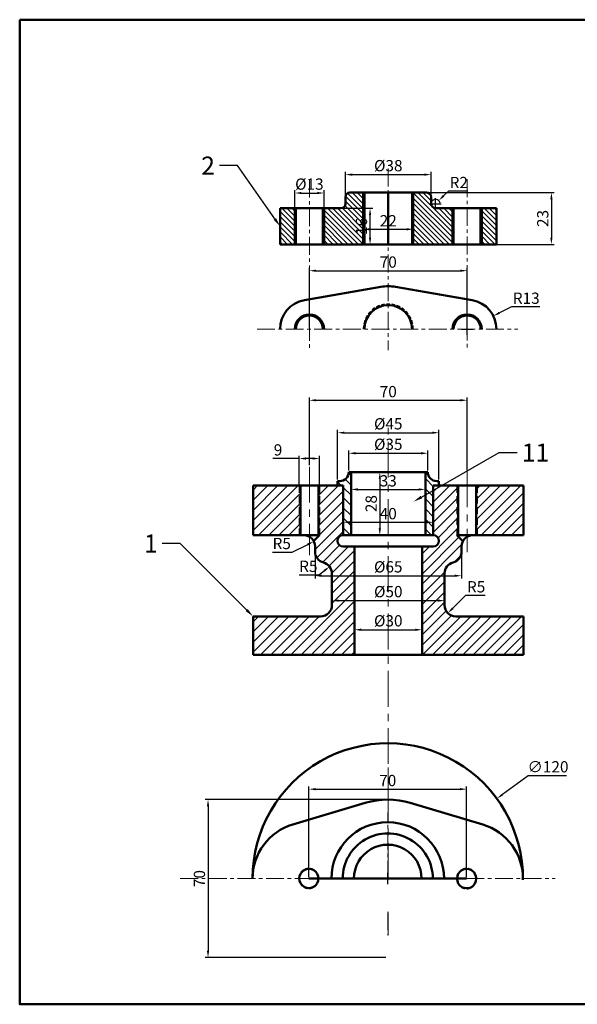
# Model space of a CAD drawing. Units: millimetres. Extents: x -656 to 85, y 134 to 571.
# Tile 1 of 5: x -656 to -409, y 134 to 571. Entities that reach past the tile are written whole.
import ezdxf
from ezdxf import colors
from ezdxf.entities.mleader import LeaderData, LeaderLine
from ezdxf.math import Vec2, Vec3

# ---------------------------------------------------------------- set-up
doc = ezdxf.new("R2010")
doc.units = ezdxf.units.MM
doc.header["$LTSCALE"] = 0.5
doc.linetypes.add('CENTER', pattern=[50.8, 31.75, -6.35, 6.35, -6.35])
doc.linetypes.add('HIDDEN', pattern=[9.525, 6.35, -3.175])
for name, color, linetype, lineweight in [('M-CNTR', 1, 'CENTER', 18), ('M-DIMS', 2, 'Continuous', 25), ('M-HATC', 8, 'Continuous', 18), ('M-HIDN', 3, 'HIDDEN', 25), ('M-OUTL', 7, 'Continuous', 50), ('M-TEXT', 7, 'Continuous', 25), ('M-TTLB', 7, 'Continuous', 50)]:
    doc.layers.add(name, color=color, linetype=linetype, lineweight=lineweight)
doc.styles.get("Standard").update_dxf_attribs({"font": 'arial.ttf'})
doc.dimstyles.new('ISO-25', dxfattribs={"dimtxt": 5, "dimasz": 3, "dimexe": 1.25, "dimexo": 0.625, "dimtad": 1, "dimtoh": 1, "dimdec": 0, "dimtxsty": 'Standard', "dimcen": 2.5, "dimadec": 0, "dimazin": 0, "dimtfac": 1, "dimtdec": 0, "dimtofl": 0, "dimtmove": 0, "dimatfit": 3, "dimfxl": 1, "dimarcsym": 0})

# ---------------------------------------------------------------- blocks, each defined once
blk = doc.blocks.new('*D1')
at = {"layer": 'Defpoints', "color": 0, "ltscale": 0.5, "transparency": 16777216}
for p in [(-475.29, 378.8), (-510.29, 370.47), (-475.29, 370.47)]:
    blk.add_point(p, dxfattribs=at)
at = {"layer": 'M-DIMS', "color": 0, "lineweight": -2, "ltscale": 0.5, "transparency": 16777216}
for p, q in [((-510.29, 371.1), (-510.29, 380.05)), ((-475.29, 371.1), (-475.29, 380.05)), ((-507.29, 378.8), (-478.29, 378.8))]:
    blk.add_line(p, q, dxfattribs=at)
at = {"layer": 'M-DIMS', "color": 0, "ltscale": 0.5, "transparency": 16777216}
for points in [[(-507.29, 379.3), (-507.29, 378.3), (-510.29, 378.8)], [(-478.29, 379.3), (-478.29, 378.3), (-475.29, 378.8)]]:
    blk.add_solid(points, dxfattribs=at)
at = {"layer": 'M-DIMS', "color": 0, "ltscale": 0.5, "transparency": 16777216, "insert": (-492.79, 382.12), "char_height": 5, "attachment_point": 5}
blk.add_mtext('%%C35', dxfattribs=at)
blk = doc.blocks.new('*D2')
at = {"layer": 'Defpoints', "color": 0, "ltscale": 0.5, "transparency": 16777216}
for p in [(-470.29, 387.9), (-515.29, 366.47), (-470.29, 366.47)]:
    blk.add_point(p, dxfattribs=at)
at = {"layer": 'M-DIMS', "color": 0, "lineweight": -2, "ltscale": 0.5, "transparency": 16777216}
for p, q in [((-515.29, 367.1), (-515.29, 389.15)), ((-470.29, 367.1), (-470.29, 389.15)), ((-512.29, 387.9), (-473.29, 387.9))]:
    blk.add_line(p, q, dxfattribs=at)
at = {"layer": 'M-DIMS', "color": 0, "ltscale": 0.5, "transparency": 16777216}
for points in [[(-512.29, 388.4), (-512.29, 387.4), (-515.29, 387.9)], [(-473.29, 388.4), (-473.29, 387.4), (-470.29, 387.9)]]:
    blk.add_solid(points, dxfattribs=at)
at = {"layer": 'M-DIMS', "color": 0, "ltscale": 0.5, "transparency": 16777216, "insert": (-492.79, 391.21), "char_height": 5, "attachment_point": 5}
blk.add_mtext('%%C45', dxfattribs=at)
blk = doc.blocks.new('*D3')
at = {"layer": 'Defpoints', "color": 0, "ltscale": 0.5, "transparency": 16777216}
for p in [(-457.79, 402.29), (-527.79, 372.84), (-457.79, 370.72)]:
    blk.add_point(p, dxfattribs=at)
at = {"layer": 'M-DIMS', "color": 0, "lineweight": -2, "ltscale": 0.5, "transparency": 16777216}
for p, q in [((-527.79, 373.47), (-527.79, 403.54)), ((-524.79, 402.29), (-460.79, 402.29)), ((-457.79, 371.34), (-457.79, 403.54))]:
    blk.add_line(p, q, dxfattribs=at)
at = {"layer": 'M-DIMS', "color": 0, "ltscale": 0.5, "transparency": 16777216}
for points in [[(-524.79, 402.79), (-524.79, 401.79), (-527.79, 402.29)], [(-460.79, 402.79), (-460.79, 401.79), (-457.79, 402.29)]]:
    blk.add_solid(points, dxfattribs=at)
at = {"layer": 'M-DIMS', "color": 0, "ltscale": 0.5, "transparency": 16777216, "insert": (-492.79, 405.47), "char_height": 5, "attachment_point": 5}
blk.add_mtext('70', dxfattribs=at)
blk = doc.blocks.new('*D4')
at = {"layer": 'Defpoints', "color": 0, "ltscale": 0.5, "transparency": 16777216}
for p in [(-523.29, 376.46), (-532.29, 364.47), (-523.29, 364.47)]:
    blk.add_point(p, dxfattribs=at)
at = {"layer": 'M-DIMS', "color": 0, "lineweight": -2, "ltscale": 0.5, "transparency": 16777216}
for p, q in [((-532.29, 376.46), (-543.97, 376.46)), ((-532.29, 365.1), (-532.29, 377.71)), ((-526.29, 376.46), (-529.29, 376.46)), ((-523.29, 365.1), (-523.29, 377.71))]:
    blk.add_line(p, q, dxfattribs=at)
at = {"layer": 'M-DIMS', "color": 0, "ltscale": 0.5, "transparency": 16777216}
for points in [[(-529.29, 376.96), (-529.29, 375.96), (-532.29, 376.46)], [(-526.29, 376.96), (-526.29, 375.96), (-523.29, 376.46)]]:
    blk.add_solid(points, dxfattribs=at)
at = {"layer": 'M-DIMS', "color": 0, "ltscale": 0.5, "transparency": 16777216, "insert": (-541.7, 379.64), "char_height": 5, "attachment_point": 5}
blk.add_mtext('9', dxfattribs=at)
blk = doc.blocks.new('*D5')
at = {"layer": 'Defpoints', "color": 0, "ltscale": 0.5, "transparency": 16777216}
for p in [(-500.43, 370.47), (-500.43, 342.47), (-496.54, 342.47)]:
    blk.add_point(p, dxfattribs=at)
at = {"layer": 'M-DIMS', "color": 0, "lineweight": -2, "ltscale": 0.5, "transparency": 16777216}
for p, q in [((-499.81, 370.47), (-495.29, 370.47)), ((-496.54, 367.47), (-496.54, 345.47)), ((-499.81, 342.47), (-495.29, 342.47))]:
    blk.add_line(p, q, dxfattribs=at)
at = {"layer": 'M-DIMS', "color": 0, "ltscale": 0.5, "transparency": 16777216}
for points in [[(-497.04, 367.47), (-496.04, 367.47), (-496.54, 370.47)], [(-497.04, 345.47), (-496.04, 345.47), (-496.54, 342.47)]]:
    blk.add_solid(points, dxfattribs=at)
at = {"layer": 'M-DIMS', "color": 0, "ltscale": 0.5, "transparency": 16777216, "insert": (-499.72, 356.47), "char_height": 5, "attachment_point": 5, "rotation": 90}
blk.add_mtext('28', dxfattribs=at)
blk = doc.blocks.new('*D6')
at = {"layer": 'Defpoints', "color": 0, "ltscale": 0.5, "transparency": 16777216}
for p in [(-476.29, 362.75), (-509.29, 353.47), (-476.29, 353.47)]:
    blk.add_point(p, dxfattribs=at)
at = {"layer": 'M-DIMS', "color": 0, "lineweight": -2, "ltscale": 0.5, "transparency": 16777216}
for p, q in [((-509.29, 354.1), (-509.29, 364)), ((-506.29, 362.75), (-479.29, 362.75)), ((-476.29, 354.1), (-476.29, 364))]:
    blk.add_line(p, q, dxfattribs=at)
at = {"layer": 'M-DIMS', "color": 0, "ltscale": 0.5, "transparency": 16777216}
for points in [[(-506.29, 363.25), (-506.29, 362.25), (-509.29, 362.75)], [(-479.29, 363.25), (-479.29, 362.25), (-476.29, 362.75)]]:
    blk.add_solid(points, dxfattribs=at)
at = {"layer": 'M-DIMS', "color": 0, "ltscale": 0.5, "transparency": 16777216, "insert": (-492.79, 365.93), "char_height": 5, "attachment_point": 5}
blk.add_mtext('33', dxfattribs=at)
blk = doc.blocks.new('*D7')
at = {"layer": 'Defpoints', "color": 0, "ltscale": 0.5, "transparency": 16777216}
for p in [(-512.79, 347.94), (-472.79, 348.2), (-472.79, 347.94)]:
    blk.add_point(p, dxfattribs=at)
at = {"layer": 'M-DIMS', "color": 0, "lineweight": -2, "ltscale": 0.5, "transparency": 16777216}
for p, q in [((-512.79, 348.56), (-512.79, 349.45)), ((-472.79, 348.56), (-472.79, 349.45)), ((-509.79, 348.2), (-475.79, 348.2))]:
    blk.add_line(p, q, dxfattribs=at)
at = {"layer": 'M-DIMS', "color": 0, "ltscale": 0.5, "transparency": 16777216}
for points in [[(-509.79, 348.7), (-509.79, 347.7), (-512.79, 348.2)], [(-475.79, 348.7), (-475.79, 347.7), (-472.79, 348.2)]]:
    blk.add_solid(points, dxfattribs=at)
at = {"layer": 'M-DIMS', "color": 0, "ltscale": 0.5, "transparency": 16777216, "insert": (-492.79, 351.38), "char_height": 5, "attachment_point": 5}
blk.add_mtext('40', dxfattribs=at)
blk = doc.blocks.new('*D8')
at = {"layer": 'Defpoints', "color": 0, "ltscale": 0.5, "transparency": 16777216}
for p in [(-525.29, 336.31), (-460.29, 336.31), (-460.29, 324.48)]:
    blk.add_point(p, dxfattribs=at)
at = {"layer": 'M-DIMS', "color": 0, "lineweight": -2, "ltscale": 0.5, "transparency": 16777216}
for p, q in [((-525.29, 335.69), (-525.29, 323.23)), ((-460.29, 335.69), (-460.29, 323.23)), ((-522.29, 324.48), (-463.29, 324.48))]:
    blk.add_line(p, q, dxfattribs=at)
at = {"layer": 'M-DIMS', "color": 0, "ltscale": 0.5, "transparency": 16777216}
for points in [[(-522.29, 324.98), (-522.29, 323.98), (-525.29, 324.48)], [(-463.29, 324.98), (-463.29, 323.98), (-460.29, 324.48)]]:
    blk.add_solid(points, dxfattribs=at)
at = {"layer": 'M-DIMS', "color": 0, "ltscale": 0.5, "transparency": 16777216, "insert": (-492.79, 327.8), "char_height": 5, "attachment_point": 5}
blk.add_mtext('%%C65', dxfattribs=at)
blk = doc.blocks.new('*D9')
at = {"layer": 'Defpoints', "color": 0, "ltscale": 0.5, "transparency": 16777216}
for p in [(-517.79, 318.47), (-467.79, 318.47), (-467.79, 313.47)]:
    blk.add_point(p, dxfattribs=at)
at = {"layer": 'M-DIMS', "color": 0, "lineweight": -2, "ltscale": 0.5, "transparency": 16777216}
for p, q in [((-517.79, 317.85), (-517.79, 312.22)), ((-467.79, 317.85), (-467.79, 312.22)), ((-514.79, 313.47), (-470.79, 313.47))]:
    blk.add_line(p, q, dxfattribs=at)
at = {"layer": 'M-DIMS', "color": 0, "ltscale": 0.5, "transparency": 16777216}
for points in [[(-514.79, 313.97), (-514.79, 312.97), (-517.79, 313.47)], [(-470.79, 313.97), (-470.79, 312.97), (-467.79, 313.47)]]:
    blk.add_solid(points, dxfattribs=at)
at = {"layer": 'M-DIMS', "color": 0, "ltscale": 0.5, "transparency": 16777216, "insert": (-492.79, 316.79), "char_height": 5, "attachment_point": 5}
blk.add_mtext('%%C50', dxfattribs=at)
blk = doc.blocks.new('*D10')
at = {"layer": 'Defpoints', "color": 0, "ltscale": 0.5, "transparency": 16777216}
for p in [(-507.79, 301.05), (-477.79, 301.05), (-477.79, 300.54)]:
    blk.add_point(p, dxfattribs=at)
at = {"layer": 'M-DIMS', "color": 0, "lineweight": -2, "ltscale": 0.5, "transparency": 16777216}
for p, q in [((-507.79, 300.43), (-507.79, 299.29)), ((-504.79, 300.54), (-480.79, 300.54)), ((-477.79, 300.43), (-477.79, 299.29))]:
    blk.add_line(p, q, dxfattribs=at)
at = {"layer": 'M-DIMS', "color": 0, "ltscale": 0.5, "transparency": 16777216}
for points in [[(-504.79, 301.04), (-504.79, 300.04), (-507.79, 300.54)], [(-480.79, 301.04), (-480.79, 300.04), (-477.79, 300.54)]]:
    blk.add_solid(points, dxfattribs=at)
at = {"layer": 'M-DIMS', "color": 0, "ltscale": 0.5, "transparency": 16777216, "insert": (-492.79, 303.86), "char_height": 5, "attachment_point": 5}
blk.add_mtext('%%C30', dxfattribs=at)
blk = doc.blocks.new('*D11')
at = {"layer": 'Defpoints', "color": 0, "ltscale": 0.5, "transparency": 16777216}
for p in [(-462.79, 311.47), (-466.33, 307.94)]:
    blk.add_point(p, dxfattribs=at)
at = {"layer": 'M-DIMS', "color": 0, "lineweight": -2, "ltscale": 0.5, "transparency": 16777216}
for p, q in [((-458.49, 315.77), (-464.2, 310.06)), ((-449.76, 315.77), (-458.49, 315.77))]:
    blk.add_line(p, q, dxfattribs=at)
at = {"layer": 'M-DIMS', "color": 0, "ltscale": 0.5, "transparency": 16777216}
blk.add_solid([(-464.56, 310.41), (-463.85, 309.7), (-466.33, 307.94)], dxfattribs=at)
at = {"layer": 'M-DIMS', "color": 0, "ltscale": 0.5, "transparency": 16777216, "insert": (-453.81, 318.94), "char_height": 5, "attachment_point": 5}
blk.add_mtext('R5', dxfattribs=at)
blk = doc.blocks.new('*D12')
at = {"layer": 'Defpoints', "color": 0, "ltscale": 0.5, "transparency": 16777216}
for p in [(-518.84, 328.53), (-522.79, 325.47)]:
    blk.add_point(p, dxfattribs=at)
at = {"layer": 'M-DIMS', "color": 0, "lineweight": -2, "ltscale": 0.5, "transparency": 16777216}
for p, q in [((-532.31, 324.86), (-523.58, 324.86)), ((-523.58, 324.86), (-521.21, 326.7))]:
    blk.add_line(p, q, dxfattribs=at)
at = {"layer": 'M-DIMS', "color": 0, "ltscale": 0.5, "transparency": 16777216}
blk.add_solid([(-521.52, 327.09), (-520.9, 326.3), (-518.84, 328.53)], dxfattribs=at)
at = {"layer": 'M-DIMS', "color": 0, "ltscale": 0.5, "transparency": 16777216, "insert": (-528.26, 328.03), "char_height": 5, "attachment_point": 5}
blk.add_mtext('R5', dxfattribs=at)
blk = doc.blocks.new('*D13')
at = {"layer": 'Defpoints', "color": 0, "ltscale": 0.5, "transparency": 16777216}
for p in [(-530.29, 337.47), (-525.81, 339.69)]:
    blk.add_point(p, dxfattribs=at)
at = {"layer": 'M-DIMS', "color": 0, "lineweight": -2, "ltscale": 0.5, "transparency": 16777216}
for p, q in [((-535.38, 334.96), (-528.5, 338.36)), ((-544.1, 334.96), (-535.38, 334.96))]:
    blk.add_line(p, q, dxfattribs=at)
at = {"layer": 'M-DIMS', "color": 0, "ltscale": 0.5, "transparency": 16777216}
blk.add_solid([(-528.72, 338.81), (-528.28, 337.91), (-525.81, 339.69)], dxfattribs=at)
at = {"layer": 'M-DIMS', "color": 0, "ltscale": 0.5, "transparency": 16777216, "insert": (-540.05, 338.13), "char_height": 5, "attachment_point": 5}
blk.add_mtext('R5', dxfattribs=at)
blk = doc.blocks.new('*D14')
at = {"layer": 'Defpoints', "color": 0, "ltscale": 0.5, "transparency": 16777216}
for p in [(-458.02, 229.87), (-528.02, 190.27), (-458.02, 190.23)]:
    blk.add_point(p, dxfattribs=at)
at = {"layer": 'M-DIMS', "color": 0, "lineweight": -2, "ltscale": 0.5, "transparency": 16777216}
for p, q in [((-528.02, 190.89), (-528.02, 231.12)), ((-525.02, 229.87), (-461.02, 229.87)), ((-458.02, 190.85), (-458.02, 231.12))]:
    blk.add_line(p, q, dxfattribs=at)
at = {"layer": 'M-DIMS', "color": 0, "ltscale": 0.5, "transparency": 16777216}
for points in [[(-525.02, 230.37), (-525.02, 229.37), (-528.02, 229.87)], [(-461.02, 230.37), (-461.02, 229.37), (-458.02, 229.87)]]:
    blk.add_solid(points, dxfattribs=at)
at = {"layer": 'M-DIMS', "color": 0, "ltscale": 0.5, "transparency": 16777216, "insert": (-493.02, 233.05), "char_height": 5, "attachment_point": 5}
blk.add_mtext('70', dxfattribs=at)
blk = doc.blocks.new('*D15')
at = {"layer": 'Defpoints', "color": 0, "ltscale": 0.5, "transparency": 16777216}
for p in [(-492.79, 225.25), (-572.76, 155.25), (-493.24, 155.25)]:
    blk.add_point(p, dxfattribs=at)
at = {"layer": 'M-DIMS', "color": 0, "lineweight": -2, "ltscale": 0.5, "transparency": 16777216}
for p, q in [((-493.41, 225.25), (-574.01, 225.25)), ((-572.76, 222.25), (-572.76, 158.25)), ((-493.87, 155.25), (-574.01, 155.25))]:
    blk.add_line(p, q, dxfattribs=at)
at = {"layer": 'M-DIMS', "color": 0, "ltscale": 0.5, "transparency": 16777216}
for points in [[(-573.26, 222.25), (-572.26, 222.25), (-572.76, 225.25)], [(-573.26, 158.25), (-572.26, 158.25), (-572.76, 155.25)]]:
    blk.add_solid(points, dxfattribs=at)
at = {"layer": 'M-DIMS', "color": 0, "ltscale": 0.5, "transparency": 16777216, "insert": (-575.94, 190.23), "char_height": 5, "attachment_point": 5, "rotation": 90}
blk.add_mtext('70', dxfattribs=at)
blk = doc.blocks.new('*D16')
at = {"layer": 'Defpoints', "color": 0, "ltscale": 0.5, "transparency": 16777216}
for p in [(-444.6, 225.7), (-541.44, 154.84)]:
    blk.add_point(p, dxfattribs=at)
at = {"layer": 'M-DIMS', "color": 0, "lineweight": -2, "ltscale": 0.5, "transparency": 16777216}
for p, q in [((-430.77, 235.82), (-442.17, 227.47)), ((-413.67, 235.82), (-430.77, 235.82)), ((-493.02, 187.77), (-493.02, 192.77)), ((-495.52, 190.27), (-490.52, 190.27))]:
    blk.add_line(p, q, dxfattribs=at)
blk.add_arc((-493.02, 190.27), 60, 34.9981, 179.3036, dxfattribs=at)
at = {"layer": 'M-DIMS', "color": 0, "ltscale": 0.5, "transparency": 16777216}
blk.add_solid([(-442.47, 227.87), (-441.88, 227.07), (-444.6, 225.7)], dxfattribs=at)
at = {"layer": 'M-DIMS', "color": 0, "ltscale": 0.5, "transparency": 16777216, "insert": (-421.91, 239.14), "char_height": 5, "attachment_point": 5}
blk.add_mtext('∅120', dxfattribs=at)
blk = doc.blocks.new('*D17')
at = {"layer": 'Defpoints', "color": 0, "ltscale": 0.5, "transparency": 16777216}
for p in [(-473.79, 502.33), (-511.79, 492.39), (-473.79, 492.39)]:
    blk.add_point(p, dxfattribs=at)
at = {"layer": 'M-DIMS', "color": 0, "lineweight": -2, "ltscale": 0.5, "transparency": 16777216}
for p, q in [((-511.79, 493.02), (-511.79, 503.58)), ((-508.79, 502.33), (-476.79, 502.33)), ((-473.79, 493.02), (-473.79, 503.58))]:
    blk.add_line(p, q, dxfattribs=at)
at = {"layer": 'M-DIMS', "color": 0, "ltscale": 0.5, "transparency": 16777216}
for points in [[(-508.79, 502.83), (-508.79, 501.83), (-511.79, 502.33)], [(-476.79, 502.83), (-476.79, 501.83), (-473.79, 502.33)]]:
    blk.add_solid(points, dxfattribs=at)
at = {"layer": 'M-DIMS', "color": 0, "ltscale": 0.5, "transparency": 16777216, "insert": (-492.79, 505.65), "char_height": 5, "attachment_point": 5}
blk.add_mtext('%%C38', dxfattribs=at)
blk = doc.blocks.new('*D18')
at = {"layer": 'Defpoints', "color": 0, "ltscale": 0.5, "transparency": 16777216}
for p in [(-521.29, 494.17), (-534.29, 487.39), (-521.29, 487.39)]:
    blk.add_point(p, dxfattribs=at)
at = {"layer": 'M-DIMS', "color": 0, "lineweight": -2, "ltscale": 0.5, "transparency": 16777216}
for p, q in [((-534.29, 488.02), (-534.29, 495.42)), ((-531.29, 494.17), (-524.29, 494.17)), ((-521.29, 488.02), (-521.29, 495.42))]:
    blk.add_line(p, q, dxfattribs=at)
at = {"layer": 'M-DIMS', "color": 0, "ltscale": 0.5, "transparency": 16777216}
for points in [[(-531.29, 494.67), (-531.29, 493.67), (-534.29, 494.17)], [(-524.29, 494.67), (-524.29, 493.67), (-521.29, 494.17)]]:
    blk.add_solid(points, dxfattribs=at)
at = {"layer": 'M-DIMS', "color": 0, "ltscale": 0.5, "transparency": 16777216, "insert": (-527.79, 497.48), "char_height": 5, "attachment_point": 5}
blk.add_mtext('%%C13', dxfattribs=at)
blk = doc.blocks.new('*D19')
at = {"layer": 'Defpoints', "color": 0, "ltscale": 0.5, "transparency": 16777216}
for p in [(-471.79, 489.39), (-470.38, 490.81)]:
    blk.add_point(p, dxfattribs=at)
at = {"layer": 'M-DIMS', "color": 0, "lineweight": -2, "ltscale": 0.5, "transparency": 16777216}
for p, q in [((-466.13, 495.05), (-468.25, 492.93)), ((-457.5, 495.05), (-466.13, 495.05)), ((-474.29, 489.39), (-469.29, 489.39)), ((-471.79, 486.89), (-471.79, 491.89))]:
    blk.add_line(p, q, dxfattribs=at)
blk.add_arc((-471.79, 489.39), 2, 9.1901, 162.0951, dxfattribs=at)
at = {"layer": 'M-DIMS', "color": 0, "ltscale": 0.5, "transparency": 16777216}
blk.add_solid([(-468.61, 493.28), (-467.9, 492.57), (-470.38, 490.81)], dxfattribs=at)
at = {"layer": 'M-DIMS', "color": 0, "ltscale": 0.5, "transparency": 16777216, "insert": (-461.5, 498.18), "char_height": 5, "attachment_point": 5}
blk.add_mtext('R2', dxfattribs=at)
blk = doc.blocks.new('*D20')
at = {"layer": 'Defpoints', "color": 0, "ltscale": 0.5, "transparency": 16777216}
for p in [(-513.79, 487.39), (-500.86, 487.39), (-444.79, 471.39)]:
    blk.add_point(p, dxfattribs=at)
at = {"layer": 'M-DIMS', "color": 0, "lineweight": -2, "ltscale": 0.5, "transparency": 16777216}
for p, q in [((-513.16, 487.39), (-499.61, 487.39)), ((-500.86, 474.39), (-500.86, 484.39)), ((-445.41, 471.39), (-502.11, 471.39))]:
    blk.add_line(p, q, dxfattribs=at)
at = {"layer": 'M-DIMS', "color": 0, "ltscale": 0.5, "transparency": 16777216}
for points in [[(-501.36, 484.39), (-500.36, 484.39), (-500.86, 487.39)], [(-501.36, 474.39), (-500.36, 474.39), (-500.86, 471.39)]]:
    blk.add_solid(points, dxfattribs=at)
at = {"layer": 'M-DIMS', "color": 0, "ltscale": 0.5, "transparency": 16777216, "insert": (-504.03, 479.39), "char_height": 5, "attachment_point": 5, "rotation": 90}
blk.add_mtext('16', dxfattribs=at)
blk = doc.blocks.new('*D21')
at = {"layer": 'Defpoints', "color": 0, "ltscale": 0.5, "transparency": 16777216}
for p in [(-475.79, 494.39), (-475.79, 471.39), (-420.4, 471.39)]:
    blk.add_point(p, dxfattribs=at)
at = {"layer": 'M-DIMS', "color": 0, "lineweight": -2, "ltscale": 0.5, "transparency": 16777216}
for p, q in [((-475.16, 494.39), (-419.15, 494.39)), ((-420.4, 491.39), (-420.4, 474.39)), ((-475.16, 471.39), (-419.15, 471.39))]:
    blk.add_line(p, q, dxfattribs=at)
at = {"layer": 'M-DIMS', "color": 0, "ltscale": 0.5, "transparency": 16777216}
for points in [[(-420.9, 491.39), (-419.9, 491.39), (-420.4, 494.39)], [(-420.9, 474.39), (-419.9, 474.39), (-420.4, 471.39)]]:
    blk.add_solid(points, dxfattribs=at)
at = {"layer": 'M-DIMS', "color": 0, "ltscale": 0.5, "transparency": 16777216, "insert": (-423.58, 482.89), "char_height": 5, "attachment_point": 5, "rotation": 90}
blk.add_mtext('23', dxfattribs=at)
blk = doc.blocks.new('*D22')
at = {"layer": 'Defpoints', "color": 0, "ltscale": 0.5, "transparency": 16777216}
for p in [(-503.89, 480.98), (-481.69, 480.98), (-481.69, 478.09)]:
    blk.add_point(p, dxfattribs=at)
at = {"layer": 'M-DIMS', "color": 0, "lineweight": -2, "ltscale": 0.5, "transparency": 16777216}
for p, q in [((-503.89, 480.35), (-503.89, 476.84)), ((-481.69, 480.35), (-481.69, 476.84)), ((-500.89, 478.09), (-484.69, 478.09))]:
    blk.add_line(p, q, dxfattribs=at)
at = {"layer": 'M-DIMS', "color": 0, "ltscale": 0.5, "transparency": 16777216}
for points in [[(-500.89, 478.59), (-500.89, 477.59), (-503.89, 478.09)], [(-484.69, 478.59), (-484.69, 477.59), (-481.69, 478.09)]]:
    blk.add_solid(points, dxfattribs=at)
at = {"layer": 'M-DIMS', "color": 0, "ltscale": 0.5, "transparency": 16777216, "insert": (-492.79, 481.22), "char_height": 5, "attachment_point": 5}
blk.add_mtext('22', dxfattribs=at)
blk = doc.blocks.new('*D23')
at = {"layer": 'Defpoints', "color": 0, "ltscale": 0.5, "transparency": 16777216}
for p in [(-457.79, 459.73), (-527.79, 433.86), (-457.79, 433.86)]:
    blk.add_point(p, dxfattribs=at)
at = {"layer": 'M-DIMS', "color": 0, "lineweight": -2, "ltscale": 0.5, "transparency": 16777216}
for p, q in [((-527.79, 434.48), (-527.79, 460.98)), ((-524.79, 459.73), (-460.79, 459.73)), ((-457.79, 434.48), (-457.79, 460.98))]:
    blk.add_line(p, q, dxfattribs=at)
at = {"layer": 'M-DIMS', "color": 0, "ltscale": 0.5, "transparency": 16777216}
for points in [[(-524.79, 460.23), (-524.79, 459.23), (-527.79, 459.73)], [(-460.79, 460.23), (-460.79, 459.23), (-457.79, 459.73)]]:
    blk.add_solid(points, dxfattribs=at)
at = {"layer": 'M-DIMS', "color": 0, "ltscale": 0.5, "transparency": 16777216, "insert": (-492.79, 462.91), "char_height": 5, "attachment_point": 5}
blk.add_mtext('70', dxfattribs=at)
blk = doc.blocks.new('*D73')
at = {"layer": 'Defpoints', "color": 0, "ltscale": 0.5, "transparency": 16777216}
for p in [(-446.17, 439.68), (-457.79, 433.86)]:
    blk.add_point(p, dxfattribs=at)
at = {"layer": 'M-DIMS', "color": 0, "lineweight": -2, "ltscale": 0.5, "transparency": 16777216}
for p, q in [((-438.16, 443.7), (-443.49, 441.03)), ((-425.58, 443.7), (-438.16, 443.7)), ((-460.29, 433.86), (-455.29, 433.86)), ((-457.79, 431.36), (-457.79, 436.36))]:
    blk.add_line(p, q, dxfattribs=at)
at = {"layer": 'M-DIMS', "color": 0, "ltscale": 0.5, "transparency": 16777216}
blk.add_solid([(-443.71, 441.48), (-443.26, 440.58), (-446.17, 439.68)], dxfattribs=at)
at = {"layer": 'M-DIMS', "color": 0, "ltscale": 0.5, "transparency": 16777216, "insert": (-431.56, 446.88), "char_height": 5, "attachment_point": 5}
blk.add_mtext('R13', dxfattribs=at)

msp = doc.modelspace()

# ---------------------------------------------------------------- hatches: boundary and pattern name
at = {"layer": 'M-HATC', "ltscale": 0.5}
h = msp.add_hatch(dxfattribs=at)
h.set_pattern_fill('ANSI31', color=256, scale=0.5, angle=90)
h.set_pattern_definition([(135, (-1573.907, -110.8691), (-1.122532, -1.122532), [])])
h.paths.add_polyline_path([(-534.29, 487.39), (-540.79, 487.39), (-540.79, 471.39), (-534.29, 471.39)])
h.paths.add_polyline_path([(-503.89, 487.39), (-521.29, 487.39), (-521.29, 471.39), (-503.89, 471.39)])
h.paths.add_polyline_path([(-464.29, 487.39), (-481.69, 487.39), (-481.69, 471.39), (-464.29, 471.39)])
h.paths.add_polyline_path([(-444.79, 487.39), (-451.29, 487.39), (-451.29, 471.39), (-444.79, 471.39)])
h.paths.add_polyline_path([(-503.89, 494.39), (-509.79, 494.39, 0.414214), (-511.79, 492.39), (-511.79, 489.39, -0.414214), (-513.79, 487.39), (-503.89, 487.39)])
h.paths.add_polyline_path([(-473.79, 492.39, 0.414214), (-475.79, 494.39), (-481.69, 494.39), (-481.69, 487.39), (-471.79, 487.39, -0.414214), (-473.79, 489.39)])
h = msp.add_hatch(dxfattribs=at)
h.set_pattern_fill('ANSI31', color=256, angle=90)
h.set_pattern_definition([(135, (-1573.907, -110.869), (-2.245064, -2.245064), [])])
h.paths.add_polyline_path([(-509.29, 370.47), (-510.29, 370.47, -0.414214), (-514.29, 366.47), (-515.29, 366.47), (-515.29, 364.47), (-512.79, 364.47), (-512.79, 342.47), (-509.29, 342.47)])
h.paths.add_polyline_path([(-472.79, 364.47), (-470.29, 364.47), (-470.29, 366.47), (-471.29, 366.47, -0.414214), (-475.29, 370.47), (-476.29, 370.47), (-476.29, 342.47), (-472.79, 342.47)])
h = msp.add_hatch(dxfattribs=at)
h.set_pattern_fill('ANSI31', color=256)
h.set_pattern_definition([(45, (-1573.907, -110.869), (-2.245064, 2.245064), [])])
h.paths.add_polyline_path([(-532.29, 364.47), (-552.79, 364.47), (-552.79, 342.47), (-532.29, 342.47)], flags=17)
h.paths.add_polyline_path([(-512.79, 364.47), (-523.29, 364.47), (-523.29, 342.47), (-525.9, 339.86, -0.12531), (-525.29, 337.47), (-525.29, 335.15, 0.341999), (-521.54, 330.31, -0.341999), (-517.79, 325.47), (-517.79, 311.47, -0.414214), (-522.79, 306.47), (-552.79, 306.47), (-552.79, 289.47), (-507.79, 289.47), (-507.79, 337.47), (-512.79, 337.47, -1), (-512.79, 342.47)])
h.paths.add_polyline_path([(-462.29, 364.47), (-472.79, 364.47), (-472.79, 342.47, -1), (-472.79, 337.47), (-477.79, 337.47), (-477.79, 289.47), (-432.79, 289.47), (-432.79, 306.47), (-462.79, 306.47, -0.414214), (-467.79, 311.47), (-467.79, 325.47, -0.341999), (-464.04, 330.31, 0.341999), (-460.29, 335.15), (-460.29, 337.47, -0.12531), (-459.68, 339.86), (-462.29, 342.47)])
h.paths.add_polyline_path([(-432.79, 364.47), (-453.29, 364.47), (-453.29, 342.47), (-432.79, 342.47)], flags=17)

# ---------------------------------------------------------------- linework, layer by layer
at = {"layer": 'M-CNTR', "ltscale": 0.5}
for p, q in [((-492.79, 504.99), (-492.79, 424.55)), ((-527.79, 500.13), (-527.79, 424.55)), ((-457.79, 500.27), (-457.79, 424.55)), ((-551, 433.86), (-435.35, 433.86)), ((-493.02, 190.23), (-492.79, 250.23)), ((-585.11, 190.23), (-418.69, 190.23)), ((-493.02, 190.27), (-493.02, 190.23)), ((-492.99, 175.25), (-492.97, 165.27))]:
    msp.add_line(p, q, dxfattribs=at)
at = {"layer": 'M-CNTR'}
for p, q in [((-492.79, 190.23), (-492.79, 390.14)), ((-527.79, 372.84), (-527.79, 333.6)), ((-457.79, 370.72), (-457.79, 334.97)), ((-492.79, 165.27), (-492.79, 175.25))]:
    msp.add_line(p, q, dxfattribs=at)
at = {"layer": 'M-HIDN'}
for p, q in [((-532.29, 364.47), (-532.29, 342.47)), ((-523.29, 364.47), (-523.29, 342.47)), ((-462.29, 364.47), (-462.29, 342.47)), ((-453.29, 364.47), (-453.29, 342.47))]:
    msp.add_line(p, q, dxfattribs=at)
at = {"layer": 'M-HIDN', "ltscale": 0.5}
for centre, radius, start, end in [((-492.79, 433.86), 11.1, 0, 180), ((-528.02, 190.25), 4.5, 359.7235, 180.2765), ((-458.02, 190.23), 4.5, 0, 180), ((-528.02, 190.31), 4.5, 179.624, 0.1769), ((-458.02, 190.21), 4.5, 179.9005, 359.9005)]:
    msp.add_arc(centre, radius, start, end, dxfattribs=at)
at = {"layer": 'M-OUTL', "ltscale": 0.5}
for p, q in [((-509.79, 494.39), (-475.79, 494.39)), ((-503.89, 471.39), (-503.89, 494.39)), ((-503.39, 471.39), (-503.39, 494.39)), ((-492.79, 471.39), (-492.79, 494.39)), ((-482.19, 471.39), (-482.19, 494.39)), ((-481.69, 471.39), (-481.69, 494.39)), ((-511.79, 492.39), (-511.79, 489.39)), ((-473.79, 492.39), (-473.79, 489.39)), ((-540.79, 487.39), (-513.79, 487.39)), ((-540.79, 487.39), (-540.79, 471.39)), ((-534.29, 487.39), (-534.29, 471.39)), ((-533.79, 487.39), (-533.79, 471.39)), ((-521.79, 487.39), (-521.79, 471.39)), ((-521.29, 487.39), (-521.29, 471.39)), ((-492.79, 471.39), (-492.79, 487.39)), ((-471.79, 487.39), (-444.79, 487.39)), ((-464.29, 487.39), (-464.29, 471.39)), ((-463.79, 487.39), (-463.79, 471.39)), ((-451.79, 487.39), (-451.79, 471.39)), ((-451.29, 487.39), (-451.29, 471.39)), ((-444.79, 471.39), (-444.79, 487.39)), ((-540.79, 471.39), (-444.79, 471.39)), ((-530.02, 446.66), (-496.05, 452.58)), ((-455.56, 446.66), (-489.53, 452.58)), ((-462.29, 342.47), (-453.29, 342.47)), ((-462.29, 342.47), (-459.68, 339.86)), ((-535.14, 214.23), (-503, 223.79)), ((-450.86, 214.18), (-483, 223.78)), ((-458.02, 190.21), (-528.02, 190.29)), ((-458.02, 190.23), (-528.02, 190.27)), ((-458.02, 190.23), (-458.02, 190.27)), ((-458.02, 190.21), (-458.02, 190.16))]:
    msp.add_line(p, q, dxfattribs=at)
at = {"layer": 'M-OUTL'}
for p, q in [((-510.29, 370.47), (-475.29, 370.47)), ((-509.29, 342.47), (-509.29, 370.47)), ((-476.29, 342.47), (-476.29, 370.47)), ((-552.79, 364.47), (-512.79, 364.47)), ((-552.79, 364.47), (-552.79, 342.47)), ((-531.79, 364.47), (-531.79, 342.47)), ((-523.79, 364.47), (-523.79, 342.47)), ((-515.29, 366.47), (-514.29, 366.47)), ((-515.29, 364.47), (-515.29, 366.47)), ((-512.79, 342.47), (-512.79, 364.47)), ((-472.79, 364.47), (-457.79, 364.47)), ((-472.79, 364.47), (-432.79, 364.47)), ((-472.79, 342.47), (-472.79, 364.47)), ((-471.29, 366.47), (-470.29, 366.47)), ((-470.29, 364.47), (-470.29, 366.47)), ((-461.79, 364.47), (-461.79, 342.47)), ((-453.79, 364.47), (-453.79, 342.47)), ((-432.79, 342.47), (-432.79, 364.47)), ((-552.79, 342.47), (-530.29, 342.47)), ((-532.29, 342.47), (-523.29, 342.47)), ((-523.29, 342.47), (-525.9, 339.86)), ((-512.79, 342.47), (-472.79, 342.47)), ((-455.29, 342.47), (-432.79, 342.47)), ((-525.29, 335.15), (-525.29, 337.47)), ((-512.79, 337.47), (-472.79, 337.47)), ((-507.79, 289.47), (-507.79, 337.47)), ((-477.79, 289.47), (-477.79, 337.47)), ((-460.29, 335.15), (-460.29, 337.47)), ((-517.79, 311.47), (-517.79, 325.47)), ((-467.79, 311.47), (-467.79, 325.47)), ((-552.79, 306.47), (-552.79, 289.47)), ((-522.79, 306.47), (-552.79, 306.47)), ((-432.79, 306.47), (-462.79, 306.47)), ((-432.79, 289.47), (-432.79, 306.47)), ((-552.79, 289.47), (-432.79, 289.47))]:
    msp.add_line(p, q, dxfattribs=at)
at = {"layer": 'M-OUTL', "ltscale": 0.5}
for centre, radius, start, end in [((-509.79, 492.39), 2, 90, 180), ((-475.79, 492.39), 2, 0, 90), ((-513.79, 489.39), 2, 270, 0), ((-471.79, 489.39), 2, 180, 270), ((-492.79, 433.86), 19, 80.1291, 99.8709), ((-527.79, 433.86), 13, 99.8709, 180), ((-457.79, 433.86), 13, 0, 80.1291), ((-492.79, 433.86), 10.6, 0, 180), ((-527.79, 433.86), 6.5, 0, 180), ((-527.79, 433.86), 6, 0, 180), ((-457.79, 433.86), 6.5, 0, 180), ((-457.79, 433.86), 6, 0, 180), ((-493.02, 190.23), 60, 359.5633, 180), ((-493.02, 190.25), 35, 73.3629, 106.566), ((-528.02, 190.27), 25, 106.566, 180.0995), ((-493.02, 190.23), 25, 0, 180), ((-458.02, 190.23), 25, 358.9519, 73.3629), ((-493.02, 190.25), 20, 359.9378, 180.0622), ((-493.02, 190.25), 15, 359.9171, 180.0829), ((-528.02, 190.27), 4.25, 359.4145, 180.5855), ((-458.02, 190.27), 4.25, 359.4145, 180.5855), ((-493.02, 190.27), 60, 179.9005, 180.0415), ((-528.02, 190.29), 25, 179.8009, 180.1394), ((-528.02, 190.29), 4.25, 179.3149, 0.486), ((-493.02, 190.25), 35, 179.8649, 179.936), ((-493.02, 190.25), 35, 179.9645, 180.0355), ((-493.02, 190.27), 25, 179.9005, 180.0995), ((-493.02, 190.25), 20, 179.8382, 180.0622), ((-493.02, 190.25), 15, 179.8175, 180.0829), ((-528.02, 190.29), 25, 359.936, 360), ((-528.02, 190.27), 25, 359.9005, 359.9645), ((-458.02, 190.21), 25, 179.9005, 179.936), ((-458.02, 190.23), 25, 179.9645, 180), ((-493.02, 190.25), 15, 359.9171, 359.9834), ((-493.02, 190.25), 20, 359.936, 359.9627), ((-493.02, 190.27), 25, 359.8862, 359.9005), ((-458.02, 190.16), 4.25, 179.3149, 0.486), ((-493.02, 190.25), 35, 359.9645, 0.0355), ((-493.02, 190.25), 35, 359.8649, 359.936), ((-458.02, 190.21), 25, 358.8523, 0.9486), ((-493.02, 190.27), 60, 359.4638, 0.3371), ((-493.02, 190.25), 15, 270.1098, 270.8641), ((-493.02, 190.25), 20, 270.112, 270.648), ((-493.02, 190.27), 25, 270.1188, 270.524)]:
    msp.add_arc(centre, radius, start, end, dxfattribs=at)
at = {"layer": 'M-OUTL'}
for centre, radius, start, end in [((-514.29, 370.47), 4, 270, 0), ((-471.29, 370.47), 4, 180, 270), ((-530.29, 337.47), 5, 0, 90), ((-512.79, 339.97), 2.5, 90, 270), ((-472.79, 339.97), 2.5, 270, 90), ((-455.29, 337.47), 5, 90, 180), ((-520.29, 335.15), 5, 180, 255.5225), ((-465.29, 335.15), 5, 284.4775, 0), ((-522.79, 325.47), 5, 0, 75.5225), ((-462.79, 325.47), 5, 104.4775, 180), ((-522.79, 311.47), 5, 270, 0), ((-462.79, 311.47), 5, 180, 270)]:
    msp.add_arc(centre, radius, start, end, dxfattribs=at)
at = {"layer": 'M-TTLB', "ltscale": 0.5}
msp.add_lwpolyline([(-656.34, 571.01), (84.63, 571.01), (84.63, 134.49), (-656.34, 134.49)], close=True, dxfattribs=at)

# ---------------------------------------------------------------- dimensions: what is measured, and where the dimension line sits
at = {"layer": 'M-DIMS', "ltscale": 0.5}
for base, p1, p2, picture, middle in [((-473.79, 502.33), (-511.79, 492.39), (-473.79, 492.39), '*D17', (-492.79, 505.65)), ((-470.29, 387.9), (-515.29, 366.47), (-470.29, 366.47), '*D2', (-492.79, 391.21)), ((-475.29, 378.8), (-510.29, 370.47), (-475.29, 370.47), '*D1', (-492.79, 382.12)), ((-467.79, 313.47), (-517.79, 318.47), (-467.79, 318.47), '*D9', (-492.79, 316.79)), ((-477.79, 300.54), (-507.79, 301.05), (-477.79, 301.05), '*D10', (-492.79, 303.86))]:
    dim = msp.add_linear_dim(base=base, p1=p1, p2=p2, text='%%C<>', dimstyle='ISO-25', override={"dimclrd": 0, "dimclre": 0, "dimclrt": 0}, dxfattribs=at)
    dim.commit()
    dim.dimension.update_dxf_attribs({"geometry": picture, "text_midpoint": middle})
for base, p1, p2, picture, middle in [((-521.29, 494.17), (-534.29, 487.39), (-521.29, 487.39), '*D18', (-527.79, 494.17)), ((-460.29, 324.48), (-525.29, 336.31), (-460.29, 336.31), '*D8', (-492.79, 324.48))]:
    dim = msp.add_linear_dim(base=base, p1=p1, p2=p2, text='%%C<>', dimstyle='ISO-25', override={"dimclrd": 0, "dimclre": 0, "dimclrt": 0}, dxfattribs=at)
    dim.commit()
    dim.dimension.update_dxf_attribs({"geometry": picture, "text_midpoint": middle, "dimtype": 160})
dim = msp.add_radius_dim(center=(-471.79, 489.39), mpoint=(-470.38, 490.81), dimstyle='ISO-25', override={"dimclrd": 0, "dimclre": 0, "dimclrt": 0}, dxfattribs=at)
dim.commit()
dim.dimension.update_dxf_attribs({"geometry": '*D19', "text_midpoint": (-461.5, 498.18)})
for base, p1, p2, picture, middle in [((-420.4, 471.39), (-475.79, 494.39), (-475.79, 471.39), '*D21', (-423.58, 482.89)), ((-500.86, 487.39), (-444.79, 471.39), (-513.79, 487.39), '*D20', (-504.03, 479.39))]:
    dim = msp.add_linear_dim(base=base, p1=p1, p2=p2, angle=90, dimstyle='ISO-25', override={"dimclrd": 0, "dimclre": 0, "dimclrt": 0}, dxfattribs=at)
    dim.commit()
    dim.dimension.update_dxf_attribs({"geometry": picture, "text_midpoint": middle})
for base, p1, p2, picture, middle in [((-481.69, 478.09), (-503.89, 480.98), (-481.69, 480.98), '*D22', (-492.79, 481.22)), ((-457.79, 459.73), (-527.79, 433.86), (-457.79, 433.86), '*D23', (-492.79, 462.91)), ((-476.29, 362.75), (-509.29, 353.47), (-476.29, 353.47), '*D6', (-492.79, 365.93)), ((-458.02, 229.87), (-528.02, 190.27), (-458.02, 190.23), '*D14', (-493.02, 233.05))]:
    dim = msp.add_linear_dim(base=base, p1=p1, p2=p2, dimstyle='ISO-25', override={"dimclrd": 0, "dimclre": 0, "dimclrt": 0}, dxfattribs=at)
    dim.commit()
    dim.dimension.update_dxf_attribs({"geometry": picture, "text_midpoint": middle})
for center, mpoint, picture, middle in [((-457.79, 433.86), (-446.17, 439.68), '*D73', (-431.56, 443.7)), ((-530.29, 337.47), (-525.81, 339.69), '*D13', (-540.05, 334.96)), ((-522.79, 325.47), (-518.84, 328.53), '*D12', (-528.26, 324.86)), ((-462.79, 311.47), (-466.33, 307.94), '*D11', (-453.81, 315.77))]:
    dim = msp.add_radius_dim(center=center, mpoint=mpoint, dimstyle='ISO-25', override={"dimclrd": 0, "dimclre": 0, "dimclrt": 0}, dxfattribs=at)
    dim.commit()
    dim.dimension.update_dxf_attribs({"geometry": picture, "text_midpoint": middle, "dimtype": 164})
for base, p1, p2, picture, middle in [((-457.79, 402.29), (-527.79, 372.84), (-457.79, 370.72), '*D3', (-492.79, 402.29)), ((-523.29, 376.46), (-532.29, 364.47), (-523.29, 364.47), '*D4', (-541.7, 376.46)), ((-472.79, 348.2), (-512.79, 347.94), (-472.79, 347.94), '*D7', (-492.79, 348.2))]:
    dim = msp.add_linear_dim(base=base, p1=p1, p2=p2, dimstyle='ISO-25', override={"dimclrd": 0, "dimclre": 0, "dimclrt": 0}, dxfattribs=at)
    dim.commit()
    dim.dimension.update_dxf_attribs({"geometry": picture, "text_midpoint": middle, "dimtype": 160})
for base, p1, p2, picture, middle in [((-496.54, 342.47), (-500.43, 370.47), (-500.43, 342.47), '*D5', (-496.54, 356.47)), ((-572.76, 155.25), (-492.79, 225.25), (-493.24, 155.25), '*D15', (-572.76, 190.23))]:
    dim = msp.add_linear_dim(base=base, p1=p1, p2=p2, angle=90, dimstyle='ISO-25', override={"dimclrd": 0, "dimclre": 0, "dimclrt": 0}, dxfattribs=at)
    dim.commit()
    dim.dimension.update_dxf_attribs({"geometry": picture, "text_midpoint": middle, "dimtype": 160})
dim = msp.add_diameter_dim_2p(p1=(-541.44, 154.84), p2=(-444.6, 225.7), dimstyle='ISO-25', override={"dimclrd": 0, "dimclre": 0, "dimclrt": 0}, dxfattribs=at)
dim.commit()
dim.dimension.update_dxf_attribs({"geometry": '*D16', "text_midpoint": (-421.91, 235.82), "dimtype": 163})

# ---------------------------------------------------------------- leaders
at = {"layer": 'M-TEXT', "ltscale": 0.5}
ml = msp.add_multileader_mtext('Standard', dxfattribs=at)
ml.set_content('2', color=256)
ml.set_leader_properties()
ml.build(insert=Vec2(0, 0))
ctx = ml.context
ctx.base_point, ctx.char_height, ctx.plane_origin = Vec3(-577.02, 506.32), 8, Vec3(-540.79, 479.39)
ctx.text_align_type = 2
notes = []
notes.append((ctx, [(0, (1, 1, 0), (-559.72, 506.32), (-1, 0), 8, [(0, [(-540.79, 479.39)], 0, [])])]))
ctx.mtext.insert, ctx.mtext.alignment, ctx.mtext.flow_direction = Vec3(-569.72, 510.32), 3, 5
ml = msp.add_multileader_mtext('Standard', dxfattribs=at)
ml.set_content('11', color=256)
ml.set_leader_properties()
ml.build(insert=Vec2(0, 0))
ctx = ml.context
ctx.base_point, ctx.char_height, ctx.plane_origin = Vec3(-435.53, 379.08), 8, Vec3(-481.56, 357.36)
notes.append((ctx, [(0, (1, 1, 0), (-443.53, 379.08), (1, 0), 8, [(0, [(-481.56, 357.36)], 0, [])])]))
ctx.mtext.insert, ctx.mtext.flow_direction = Vec3(-433.53, 383.08), 5
ml = msp.add_multileader_mtext('Standard', dxfattribs=at)
ml.set_content('1', color=256)
ml.set_leader_properties()
ml.build(insert=Vec2(0, 0))
ctx = ml.context
ctx.base_point, ctx.char_height, ctx.plane_origin = Vec3(-600.05, 338.79), 8, Vec3(-552.79, 306.47)
ctx.text_align_type = 2
notes.append((ctx, [(0, (1, 1, 0), (-585.11, 338.79), (-1, 0), 8, [(0, [(-552.79, 306.47)], 0, [])])]))
ctx.mtext.insert, ctx.mtext.alignment, ctx.mtext.flow_direction = Vec3(-595.11, 342.79), 3, 5
for ctx, leaders in notes:
    for number, flags, end, landing, length, lines in leaders:
        leader = LeaderData()
        leader.index, (leader.has_last_leader_line, leader.has_dogleg_vector, leader.attachment_direction) = number, flags
        leader.last_leader_point, leader.dogleg_vector, leader.dogleg_length = Vec3(end), Vec3(landing), length
        for number, points, colour, breaks in lines:
            line = LeaderLine()
            line.index, line.vertices, line.color, line.breaks = number, Vec3.list(points), colors.encode_raw_color(colour), breaks
            leader.lines.append(line)
        ctx.leaders.append(leader)

doc.saveas('drawing.dxf')
